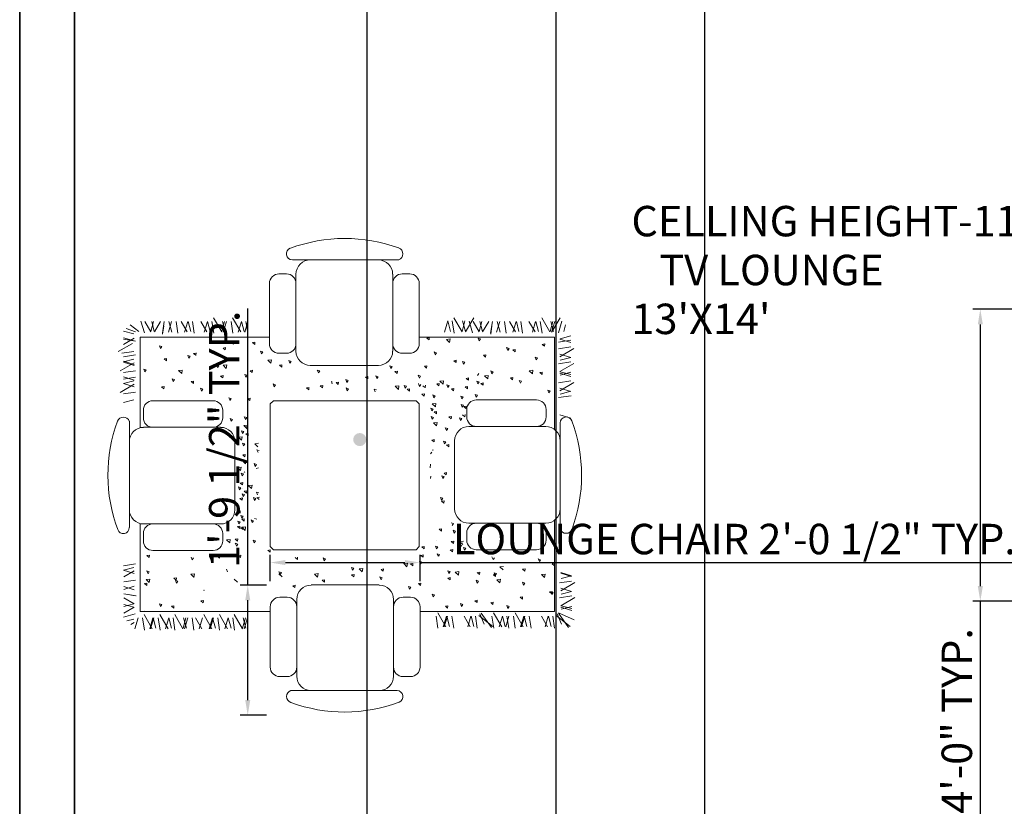
# Model space of a CAD drawing. Units: inches. Extents: x 1265 to 2734, y 1741 to 2595.
# Tile 3 of 10: x 2329 to 2490, y 2165 to 2294. Entities that reach past the tile are written whole.
import ezdxf

# ---------------------------------------------------------------- set-up
doc = ezdxf.new("R2010")
doc.units = ezdxf.units.IN
doc.header["$LTSCALE"] = 0.1
for name, color, linetype, lineweight in [('A-ANNO-DIMS', 2, 'Continuous', 18), ('A-ANNO-TEXT', 7, 'Continuous', 18), ('A-AREA-IDEN', 7, 'Continuous', 18), ('A-FURN-PATT', 252, 'Continuous', 13), ('A-WALL', 7, 'Continuous', 35), ('C-PROP', 7, 'Continuous', 35), ('Furniture', 8, 'Continuous', 15)]:
    doc.layers.add(name, color=color, linetype=linetype, lineweight=lineweight)
doc.styles.get("Standard").update_dxf_attribs({"font": 'arial.ttf', "height": 5})
doc.dimstyles.new('ISO-25', dxfattribs={"dimtxt": 5, "dimasz": 2.5, "dimexe": 1.25, "dimexo": 0.625, "dimtad": 1, "dimlunit": 3, "dimtxsty": 'Standard', "dimcen": 2.5, "dimadec": 0, "dimazin": 0, "dimtfac": 1, "dimtmove": 0, "dimatfit": 3, "dimfxl": 1, "dimarcsym": 0})

# ---------------------------------------------------------------- blocks, each defined once
blk = doc.blocks.new('CHAIR-LOUNGE')
for p, q in [((6.72, 20.87), (17.9, 20.87)), ((1.57, 18.86), (2.79, 18.86)), ((4.36, 5.87), (4.36, 18.51)), ((20.25, 18.51), (20.25, 5.87)), ((21.82, 18.86), (23.04, 18.86)), ((0, 7.39), (0, 17.29)), ((4.36, 17.29), (4.36, 7.39)), ((20.25, 7.39), (20.25, 17.29)), ((24.61, 17.29), (24.61, 7.39)), ((2.79, 5.82), (1.57, 5.82)), ((23.04, 5.82), (21.82, 5.82)), ((3.38, 3.52), (20.25, 3.52)), ((17.9, 3.52), (6.72, 3.52)), ((20.25, 3.52), (20.84, 3.52))]:
    blk.add_line(p, q)
for centre, radius, start, end in [((6.72, 18.51), 2.35, 90, 180), ((17.9, 18.51), 2.35, 0, 90), ((1.57, 17.29), 1.57, 90, 180), ((2.79, 17.29), 1.57, 0, 90), ((21.82, 17.29), 1.57, 90, 180), ((23.04, 17.29), 1.57, 0, 90), ((1.57, 7.39), 1.57, 180, 270), ((2.79, 7.39), 1.57, 270, 0), ((21.82, 7.39), 1.57, 180, 270), ((23.04, 7.39), 1.57, 270, 0), ((6.72, 5.87), 2.35, 180, 270), ((17.9, 5.87), 2.35, 270, 0), ((3.74, 2.54), 1.04, 110.0456, 249.9544), ((20.84, 2.53), 0.986, 290.3611, 90), ((12.21, 25.77), 25.77, 249.9544, 290.3611)]:
    blk.add_arc(centre, radius, start, end)
blk = doc.blocks.new('*D32')
at = {"layer": 'A-ANNO-DIMS', "color": 0, "lineweight": -2, "transparency": 16777216}
for p, q in [((2369.76, 2201.71), (2369.76, 2206.02)), ((2372.26, 2204.77), (2391.87, 2204.77)), ((2394.37, 2201.71), (2394.37, 2206.02)), ((2394.37, 2204.77), (2495.13, 2204.77))]:
    blk.add_line(p, q, dxfattribs=at)
at = {"layer": 'A-ANNO-DIMS', "color": 0, "lineweight": 100, "transparency": 16777216}
for points in [[(2372.26, 2205.19), (2372.26, 2204.36), (2369.76, 2204.77)], [(2391.87, 2205.19), (2391.87, 2204.36), (2394.37, 2204.77)]]:
    blk.add_solid(points, dxfattribs=at)
at = {"layer": 'Defpoints', "color": 0, "lineweight": 100, "transparency": 16777216}
for p in [(2394.37, 2204.77), (2369.76, 2201.08), (2394.37, 2201.08)]:
    blk.add_point(p, dxfattribs=at)
at = {"layer": 'A-ANNO-DIMS', "color": 0, "transparency": 16777216, "insert": (2446, 2207.99), "char_height": 5, "attachment_point": 5}
blk.add_mtext('LOUNGE CHAIR 2\'-0 1/2" TYP.', dxfattribs=at)
blk = doc.blocks.new('*D33')
at = {"layer": 'A-ANNO-DIMS', "color": 0, "lineweight": -2, "transparency": 16777216}
for p, q in [((2366.06, 2201.08), (2366.06, 2246.49)), ((2369.13, 2201.08), (2364.81, 2201.08)), ((2366.06, 2182.18), (2366.06, 2198.58)), ((2369.13, 2179.68), (2364.81, 2179.68))]:
    blk.add_line(p, q, dxfattribs=at)
at = {"layer": 'A-ANNO-DIMS', "color": 0, "lineweight": 100, "transparency": 16777216}
for points in [[(2365.65, 2198.58), (2366.48, 2198.58), (2366.06, 2201.08)], [(2365.65, 2182.18), (2366.48, 2182.18), (2366.06, 2179.68)]]:
    blk.add_solid(points, dxfattribs=at)
at = {"layer": 'Defpoints', "color": 0, "lineweight": 100, "transparency": 16777216}
for p in [(2366.06, 2201.08), (2369.76, 2201.08), (2369.76, 2179.68)]:
    blk.add_point(p, dxfattribs=at)
at = {"layer": 'A-ANNO-DIMS', "color": 0, "transparency": 16777216, "insert": (2362.85, 2225.04), "char_height": 5, "attachment_point": 5, "rotation": 90}
blk.add_mtext('1\'-9 1/2" TYP.', dxfattribs=at)
blk = doc.blocks.new('*D36')
at = {"layer": 'A-ANNO-DIMS', "color": 0, "lineweight": -2, "transparency": 16777216}
for p, q in [((2492.98, 2246.41), (2485.15, 2246.41)), ((2486.4, 2243.91), (2486.4, 2200.91)), ((2492.98, 2198.41), (2485.15, 2198.41)), ((2486.4, 2198.41), (2486.4, 2131.39))]:
    blk.add_line(p, q, dxfattribs=at)
at = {"layer": 'A-ANNO-DIMS', "color": 0, "lineweight": 100, "transparency": 16777216}
for points in [[(2485.99, 2243.91), (2486.82, 2243.91), (2486.4, 2246.41)], [(2485.99, 2200.91), (2486.82, 2200.91), (2486.4, 2198.41)]]:
    blk.add_solid(points, dxfattribs=at)
at = {"layer": 'Defpoints', "color": 0, "lineweight": 100, "transparency": 16777216}
for p in [(2493.6, 2246.41), (2486.4, 2198.41), (2493.6, 2198.41)]:
    blk.add_point(p, dxfattribs=at)
at = {"layer": 'A-ANNO-DIMS', "color": 0, "transparency": 16777216, "insert": (2483.19, 2163.65), "char_height": 5, "attachment_point": 5, "rotation": 90}
blk.add_mtext('WINDOW 4\'-0" TYP.', dxfattribs=at)
blk = doc.blocks.new('*D42')
at = {"layer": 'A-ANNO-DIMS', "color": 0, "lineweight": -2, "transparency": 16777216}
for p, q in [((2328.6, 1822.68), (2328.6, 2585.16)), ((2521.32, 1822.68), (2521.32, 2585.16)), ((2331.1, 2583.91), (2518.82, 2583.91))]:
    blk.add_line(p, q, dxfattribs=at)
at = {"layer": 'A-ANNO-DIMS', "color": 0, "lineweight": 100, "transparency": 16777216}
for points in [[(2331.1, 2584.32), (2331.1, 2583.49), (2328.6, 2583.91)], [(2518.82, 2584.32), (2518.82, 2583.49), (2521.32, 2583.91)]]:
    blk.add_solid(points, dxfattribs=at)
at = {"layer": 'Defpoints', "color": 0, "lineweight": 100, "transparency": 16777216}
for p in [(2521.32, 2583.91), (2328.6, 1822.06), (2521.32, 1822.06)]:
    blk.add_point(p, dxfattribs=at)
at = {"layer": 'A-ANNO-DIMS', "color": 0, "transparency": 16777216, "insert": (2424.96, 2587.12), "char_height": 5, "attachment_point": 5}
blk.add_mtext('16\'-0 1/2"', dxfattribs=at)
blk = doc.blocks.new('*D43')
at = {"layer": 'A-ANNO-DIMS', "color": 0, "lineweight": -2, "transparency": 16777216}
for p, q in [((2337.6, 2308.03), (2337.6, 1744.16)), ((2441.1, 2308.03), (2441.1, 1744.16)), ((2340.1, 1745.41), (2438.6, 1745.41))]:
    blk.add_line(p, q, dxfattribs=at)
at = {"layer": 'A-ANNO-DIMS', "color": 0, "lineweight": 100, "transparency": 16777216}
for points in [[(2340.1, 1745.82), (2340.1, 1744.99), (2337.6, 1745.41)], [(2438.6, 1745.82), (2438.6, 1744.99), (2441.1, 1745.41)]]:
    blk.add_solid(points, dxfattribs=at)
at = {"layer": 'Defpoints', "color": 0, "lineweight": 100, "transparency": 16777216}
for p in [(2337.6, 2308.66), (2441.1, 2308.66), (2441.1, 1745.41)]:
    blk.add_point(p, dxfattribs=at)
at = {"layer": 'A-ANNO-DIMS', "color": 0, "transparency": 16777216, "insert": (2389.35, 1748.62), "char_height": 5, "attachment_point": 5}
blk.add_mtext('8\'-7 1/2"', dxfattribs=at)
blk = doc.blocks.new('*D45')
at = {"layer": 'A-ANNO-DIMS', "color": 0, "lineweight": -2, "transparency": 16777216}
for p, q in [((2416.67, 2477.91), (2416.67, 1744.16)), ((2385.6, 2477.53), (2385.6, 1744.16)), ((2388.1, 1745.41), (2414.17, 1745.41))]:
    blk.add_line(p, q, dxfattribs=at)
at = {"layer": 'A-ANNO-DIMS', "color": 0, "lineweight": 100, "transparency": 16777216}
for points in [[(2388.1, 1745.82), (2388.1, 1744.99), (2385.6, 1745.41)], [(2414.17, 1745.82), (2414.17, 1744.99), (2416.67, 1745.41)]]:
    blk.add_solid(points, dxfattribs=at)
at = {"layer": 'Defpoints', "color": 0, "lineweight": 100, "transparency": 16777216}
for p in [(2385.6, 2478.16), (2416.67, 2478.54), (2416.67, 1745.41)]:
    blk.add_point(p, dxfattribs=at)
at = {"layer": 'A-ANNO-DIMS', "color": 0, "transparency": 16777216, "insert": (2401.14, 1748.54), "char_height": 5, "attachment_point": 5}
blk.add_mtext('2\'-7"', dxfattribs=at)

msp = doc.modelspace()

# ---------------------------------------------------------------- hatches: boundary and pattern name
at = {"layer": 'A-FURN-PATT'}
msp.add_hatch(color=256, dxfattribs=at).paths.add_polyline_path([(2385.543, 2224.98, 1), (2383.383, 2224.98, 1)])

# ---------------------------------------------------------------- linework, layer by layer
at = {"layer": 'A-WALL'}
msp.add_line((2337.602, 2140.657), (2337.602, 2308.657), dxfattribs=at)
at = {"layer": 'C-PROP'}
msp.add_line((2328.602, 1786.657), (2328.602, 2542.657), dxfattribs=at)
at = {"layer": 'Furniture'}
for p, q in [((2360.445, 2244.981), (2361.794, 2242.659)), ((2363.57, 2244.981), (2364.919, 2242.659)), ((2399.915, 2244.981), (2401.264, 2242.659)), ((2403.197, 2244.981), (2401.847, 2242.659)), ((2414.364, 2244.981), (2415.714, 2242.659)), ((2417.379, 2244.981), (2416.03, 2242.659)), ((2346.729, 2243.841), (2348.199, 2242.736)), ((2348.501, 2244.434), (2349.08, 2242.515)), ((2349.158, 2244.364), (2350.149, 2242.659)), ((2350.594, 2244.368), (2350.165, 2242.736)), ((2350.287, 2244.367), (2350.716, 2242.736)), ((2351.727, 2244.371), (2350.732, 2242.659)), ((2352.333, 2244.373), (2352.042, 2242.444)), ((2352.254, 2243.646), (2352.051, 2242.304)), ((2353.545, 2244.376), (2353.026, 2242.655)), ((2353.092, 2244.375), (2353.611, 2242.655)), ((2354.303, 2244.378), (2354.595, 2242.444)), ((2355.135, 2244.38), (2356.135, 2242.659)), ((2356.223, 2244.383), (2355.702, 2242.655)), ((2356.269, 2244.383), (2356.702, 2242.736)), ((2356.978, 2244.385), (2357.271, 2242.444)), ((2358.343, 2244.389), (2359.348, 2242.659)), ((2359.439, 2244.392), (2358.915, 2242.655)), ((2359.48, 2244.392), (2359.915, 2242.736)), ((2360.19, 2244.394), (2360.484, 2242.444)), ((2362.248, 2244.399), (2361.81, 2242.736)), ((2361.924, 2244.398), (2362.361, 2242.736)), ((2362.567, 2244.4), (2362.04, 2242.655)), ((2363.314, 2244.402), (2363.609, 2242.444)), ((2365.014, 2244.406), (2364.486, 2242.655)), ((2365.047, 2244.406), (2365.486, 2242.736)), ((2366.102, 2244.409), (2365.573, 2242.655)), ((2365.758, 2244.408), (2366.055, 2242.444)), ((2398.941, 2244.497), (2398.385, 2242.655)), ((2398.922, 2244.497), (2399.385, 2242.736)), ((2399.644, 2244.499), (2399.954, 2242.444)), ((2401.745, 2244.504), (2401.28, 2242.736)), ((2401.366, 2244.503), (2401.831, 2242.736)), ((2402.421, 2244.434), (2403, 2242.515)), ((2403.078, 2244.364), (2404.069, 2242.659)), ((2404.514, 2244.368), (2404.085, 2242.736)), ((2404.207, 2244.367), (2404.636, 2242.736)), ((2405.647, 2244.371), (2404.652, 2242.659)), ((2406.253, 2244.373), (2405.962, 2242.444)), ((2406.173, 2243.646), (2405.971, 2242.304)), ((2407.465, 2244.376), (2406.945, 2242.655)), ((2407.012, 2244.375), (2407.531, 2242.655)), ((2408.223, 2244.378), (2408.514, 2242.444)), ((2409.055, 2244.38), (2410.055, 2242.659)), ((2410.143, 2244.383), (2409.622, 2242.655)), ((2410.188, 2244.383), (2410.622, 2242.736)), ((2410.898, 2244.385), (2411.191, 2242.444)), ((2412.263, 2244.389), (2413.268, 2242.659)), ((2413.359, 2244.392), (2412.835, 2242.655)), ((2413.399, 2244.392), (2413.835, 2242.736)), ((2414.11, 2244.394), (2414.404, 2242.444)), ((2416.167, 2244.399), (2415.73, 2242.736)), ((2415.844, 2244.398), (2416.281, 2242.736)), ((2416.486, 2244.4), (2415.96, 2242.655)), ((2417.678, 2244.434), (2417.099, 2242.515)), ((2418.27, 2243.841), (2417.979, 2242.736)), ((2345.638, 2242.806), (2347.329, 2242.361)), ((2345.638, 2241.719), (2347.409, 2241.184)), ((2346.12, 2243.232), (2347.632, 2242.659)), ((2348.415, 2226.932), (2348.415, 2241.805)), ((2348.415, 2241.805), (2369.627, 2241.805)), ((2394.237, 2241.805), (2416.453, 2241.805)), ((2395.892, 2241.73), (2395.489, 2241.656)), ((2395.857, 2241.348), (2395.89, 2241.732)), ((2406.546, 2241.802), (2406.542, 2241.805)), ((2406.546, 2241.801), (2406.546, 2241.805)), ((2416.453, 2241.805), (2416.453, 2226.644)), ((2419.139, 2242.007), (2417.402, 2241.55)), ((2344.802, 2239.433), (2347.123, 2240.783)), ((2345.636, 2241.471), (2347.621, 2241.171)), ((2345.641, 2240.592), (2347.406, 2241.618)), ((2351.957, 2240.253), (2351.568, 2240.384)), ((2351.742, 2239.934), (2351.569, 2240.385)), ((2351.741, 2239.933), (2351.957, 2240.253)), ((2363.665, 2240.644), (2363.492, 2241.094)), ((2363.881, 2240.963), (2363.492, 2241.093)), ((2363.665, 2240.643), (2363.881, 2240.963)), ((2367.219, 2240.607), (2366.849, 2240.918)), ((2367.254, 2240.989), (2366.85, 2240.915)), ((2367.219, 2240.606), (2367.252, 2240.991)), ((2395.857, 2241.349), (2395.487, 2241.659)), ((2399.301, 2241.521), (2398.689, 2241.45)), ((2399.212, 2240.949), (2398.69, 2241.45)), ((2399.212, 2240.948), (2399.301, 2241.521)), ((2404.102, 2241.207), (2403.929, 2241.658)), ((2404.317, 2241.526), (2403.929, 2241.656)), ((2404.102, 2241.206), (2404.318, 2241.526)), ((2414.815, 2240.305), (2414.445, 2240.615)), ((2414.85, 2240.686), (2414.446, 2240.612)), ((2414.814, 2240.304), (2414.848, 2240.688)), ((2419.141, 2241.288), (2417.111, 2240.981)), ((2419.144, 2240.201), (2417.111, 2239.894)), ((2419.142, 2240.914), (2417.322, 2241.464)), ((2345.371, 2239.176), (2347.338, 2239.473)), ((2345.647, 2238.585), (2347.621, 2238.883)), ((2356.408, 2238.368), (2356.235, 2238.819)), ((2356.623, 2238.687), (2356.235, 2238.818)), ((2356.408, 2238.367), (2356.624, 2238.688)), ((2357.538, 2238.822), (2357.168, 2239.132)), ((2357.573, 2239.203), (2357.17, 2239.129)), ((2357.538, 2238.82), (2357.571, 2239.205)), ((2362.378, 2239.715), (2362.009, 2240.025)), ((2362.413, 2240.096), (2362.01, 2240.022)), ((2362.378, 2239.713), (2362.412, 2240.098)), ((2368.547, 2239.397), (2368.158, 2239.527)), ((2368.332, 2239.078), (2368.159, 2239.529)), ((2368.331, 2239.077), (2368.547, 2239.397)), ((2397.06, 2239.25), (2396.671, 2239.381)), ((2396.845, 2238.932), (2396.672, 2239.382)), ((2396.844, 2238.931), (2397.06, 2239.251)), ((2405.134, 2238.519), (2404.764, 2238.83)), ((2405.169, 2238.9), (2404.766, 2238.826)), ((2405.134, 2238.518), (2405.167, 2238.903)), ((2408.984, 2239.96), (2408.595, 2240.091)), ((2408.769, 2239.641), (2408.596, 2240.092)), ((2408.768, 2239.64), (2408.984, 2239.96)), ((2409.974, 2239.412), (2409.605, 2239.722)), ((2410.009, 2239.793), (2409.606, 2239.719)), ((2409.974, 2239.411), (2410.008, 2239.795)), ((2413.65, 2238.394), (2413.261, 2238.525)), ((2413.435, 2238.076), (2413.262, 2238.526)), ((2419.149, 2238.466), (2417.322, 2239.018)), ((2419.647, 2239.934), (2417.326, 2238.585)), ((2345.084, 2236.262), (2347.406, 2237.611)), ((2345.649, 2237.736), (2347.329, 2238.178)), ((2345.649, 2237.845), (2347.409, 2237.314)), ((2345.649, 2237.709), (2347.409, 2237.178)), ((2352.698, 2237.929), (2352.328, 2238.239)), ((2352.733, 2238.31), (2352.329, 2238.236)), ((2352.697, 2237.928), (2352.731, 2238.312)), ((2361.29, 2237.122), (2360.901, 2237.252)), ((2361.075, 2236.803), (2360.902, 2237.253)), ((2361.074, 2236.802), (2361.29, 2237.122)), ((2362.633, 2237.255), (2362.022, 2237.184)), ((2362.544, 2236.683), (2362.022, 2237.184)), ((2362.544, 2236.683), (2362.633, 2237.255)), ((2369.966, 2238.108), (2369.355, 2238.037)), ((2369.878, 2237.536), (2369.356, 2238.037)), ((2369.878, 2237.536), (2369.967, 2238.108)), ((2371.655, 2236.885), (2371.286, 2237.195)), ((2371.69, 2237.266), (2371.287, 2237.192)), ((2371.655, 2236.884), (2371.689, 2237.268)), ((2373.213, 2237.831), (2372.824, 2237.962)), ((2372.998, 2237.512), (2372.825, 2237.963)), ((2372.997, 2237.511), (2373.213, 2237.831)), ((2389.803, 2236.975), (2389.414, 2237.106)), ((2389.588, 2236.656), (2389.415, 2237.107)), ((2389.587, 2236.655), (2389.803, 2236.975)), ((2395.453, 2236.734), (2395.084, 2237.044)), ((2395.488, 2237.115), (2395.085, 2237.04)), ((2395.453, 2236.732), (2395.487, 2237.117)), ((2400.294, 2237.626), (2399.924, 2237.937)), ((2400.329, 2238.008), (2399.925, 2237.933)), ((2400.293, 2237.625), (2400.327, 2238.01)), ((2401.727, 2237.685), (2401.338, 2237.815)), ((2401.512, 2237.366), (2401.339, 2237.816)), ((2401.511, 2237.365), (2401.727, 2237.685)), ((2413.434, 2238.075), (2413.65, 2238.395)), ((2419.151, 2237.757), (2417.111, 2237.449)), ((2419.647, 2237.488), (2417.326, 2236.139)), ((2419.149, 2238.477), (2417.402, 2238.018)), ((2345.654, 2236.004), (2347.621, 2236.301)), ((2345.656, 2235.262), (2347.409, 2234.732)), ((2349.366, 2236.412), (2348.977, 2236.542)), ((2349.151, 2236.093), (2348.978, 2236.544)), ((2349.15, 2236.092), (2349.366, 2236.412)), ((2355.299, 2236.402), (2354.688, 2236.331)), ((2355.211, 2235.83), (2354.689, 2236.331)), ((2355.211, 2235.83), (2355.3, 2236.402)), ((2361.975, 2235.099), (2361.605, 2235.409)), ((2362.01, 2235.481), (2361.606, 2235.406)), ((2361.974, 2235.098), (2362.008, 2235.482)), ((2365.956, 2235.556), (2365.567, 2235.686)), ((2365.741, 2235.237), (2365.568, 2235.687)), ((2365.74, 2235.236), (2365.956, 2235.556)), ((2366.815, 2235.992), (2366.445, 2236.302)), ((2366.85, 2236.373), (2366.447, 2236.299)), ((2366.815, 2235.991), (2366.848, 2236.375)), ((2377.664, 2235.947), (2377.491, 2236.397)), ((2377.88, 2236.265), (2377.491, 2236.396)), ((2377.664, 2235.946), (2377.88, 2236.266)), ((2385.773, 2234.948), (2385.403, 2235.258)), ((2385.807, 2235.329), (2385.404, 2235.255)), ((2385.772, 2234.947), (2385.806, 2235.331)), ((2387.499, 2235.314), (2387.11, 2235.445)), ((2387.284, 2234.995), (2387.111, 2235.446)), ((2387.283, 2234.994), (2387.499, 2235.314)), ((2390.613, 2235.841), (2390.243, 2236.151)), ((2390.648, 2236.222), (2390.244, 2236.148)), ((2390.613, 2235.839), (2390.646, 2236.224)), ((2394.469, 2235.409), (2394.08, 2235.54)), ((2394.254, 2235.091), (2394.081, 2235.541)), ((2394.254, 2235.09), (2394.469, 2235.41)), ((2403.825, 2235.507), (2404.041, 2235.827)), ((2405.569, 2235.506), (2404.958, 2235.435)), ((2405.481, 2234.934), (2404.958, 2235.435)), ((2405.481, 2234.934), (2405.569, 2235.506)), ((2406.393, 2236.119), (2406.004, 2236.249)), ((2406.178, 2235.8), (2406.005, 2236.251)), ((2406.177, 2235.799), (2406.393, 2236.119)), ((2412.902, 2236.359), (2412.291, 2236.288)), ((2412.814, 2235.787), (2412.292, 2236.288)), ((2412.814, 2235.787), (2412.903, 2236.359)), ((2414.411, 2235.689), (2414.041, 2236)), ((2414.446, 2236.071), (2414.042, 2235.996)), ((2414.411, 2235.688), (2414.444, 2236.073)), ((2419.157, 2235.339), (2417.322, 2235.893)), ((2419.156, 2235.661), (2417.402, 2236.122)), ((2419.155, 2236.033), (2417.402, 2235.572)), ((2345.084, 2232.729), (2347.406, 2234.079)), ((2345.657, 2234.918), (2347.621, 2235.214)), ((2345.658, 2234.206), (2347.329, 2234.645)), ((2345.658, 2234.174), (2347.409, 2233.645)), ((2352.329, 2233.695), (2351.926, 2233.621)), ((2352.294, 2233.312), (2352.327, 2233.697)), ((2353.817, 2234.527), (2353.644, 2234.978)), ((2354.033, 2234.846), (2353.644, 2234.977)), ((2353.817, 2234.526), (2354.033, 2234.846)), ((2357.134, 2234.206), (2356.765, 2234.516)), ((2357.169, 2234.588), (2356.766, 2234.513)), ((2357.134, 2234.205), (2357.168, 2234.59)), ((2370.622, 2233.99), (2370.233, 2234.121)), ((2370.407, 2233.671), (2370.234, 2234.122)), ((2370.407, 2233.67), (2370.622, 2233.99)), ((2378.344, 2233.478), (2377.974, 2233.788)), ((2378.379, 2233.86), (2377.975, 2233.785)), ((2378.344, 2233.477), (2378.377, 2233.861)), ((2379.957, 2234.487), (2379.805, 2234.538)), ((2379.957, 2234.145), (2379.806, 2234.539)), ((2380.932, 2234.055), (2380.563, 2234.365)), ((2380.967, 2234.436), (2380.564, 2234.362)), ((2380.932, 2234.054), (2380.966, 2234.438)), ((2382.546, 2234.7), (2382.157, 2234.83)), ((2382.331, 2234.381), (2382.158, 2234.831)), ((2382.33, 2234.38), (2382.546, 2234.7)), ((2390.902, 2233.8), (2390.291, 2233.729)), ((2390.814, 2233.228), (2390.291, 2233.729)), ((2390.813, 2233.227), (2390.902, 2233.8)), ((2392.165, 2233.748), (2391.776, 2233.879)), ((2391.95, 2233.43), (2391.777, 2233.88)), ((2391.95, 2233.429), (2392.165, 2233.749)), ((2394.302, 2233.722), (2394.129, 2234.172)), ((2394.302, 2233.721), (2394.517, 2234.041)), ((2395.216, 2233.509), (2394.846, 2233.819)), ((2395.215, 2233.508), (2395.249, 2233.893)), ((2397.468, 2233.825), (2397.098, 2234.135)), ((2397.502, 2234.206), (2397.099, 2234.132)), ((2397.467, 2233.824), (2397.501, 2234.209)), ((2398.235, 2234.653), (2397.624, 2234.582)), ((2398.147, 2234.081), (2397.625, 2234.582)), ((2398.147, 2234.081), (2398.236, 2234.653)), ((2399.136, 2233.844), (2398.747, 2233.974)), ((2398.921, 2233.525), (2398.748, 2233.975)), ((2398.92, 2233.524), (2399.136, 2233.844)), ((2402.142, 2233.327), (2401.772, 2233.637)), ((2402.177, 2233.708), (2401.773, 2233.634)), ((2402.308, 2234.718), (2401.938, 2235.028)), ((2402.343, 2235.099), (2401.939, 2235.025)), ((2402.141, 2233.326), (2402.175, 2233.71)), ((2402.308, 2234.717), (2402.341, 2235.101)), ((2404.089, 2234.458), (2403.7, 2234.588)), ((2403.874, 2234.139), (2403.701, 2234.59)), ((2403.873, 2234.138), (2404.089, 2234.458)), ((2404.73, 2233.904), (2404.36, 2234.214)), ((2404.765, 2234.285), (2404.362, 2234.211)), ((2404.73, 2233.902), (2404.763, 2234.287)), ((2409.57, 2234.797), (2409.201, 2235.107)), ((2409.605, 2235.178), (2409.202, 2235.103)), ((2409.57, 2234.795), (2409.604, 2235.18)), ((2411.059, 2234.553), (2410.67, 2234.684)), ((2410.844, 2234.234), (2410.671, 2234.685)), ((2410.843, 2234.233), (2411.059, 2234.554)), ((2419.159, 2234.633), (2417.111, 2234.324)), ((2419.647, 2234.363), (2417.326, 2233.014)), ((2345.663, 2232.473), (2347.621, 2232.769)), ((2352.294, 2233.313), (2351.924, 2233.623)), ((2358.699, 2233.281), (2358.31, 2233.411)), ((2358.484, 2232.962), (2358.311, 2233.412)), ((2358.483, 2232.961), (2358.699, 2233.281)), ((2376.092, 2233.162), (2375.722, 2233.472)), ((2376.127, 2233.544), (2375.723, 2233.469)), ((2376.092, 2233.161), (2376.125, 2233.545)), ((2382.594, 2233.331), (2382.205, 2233.461)), ((2382.379, 2233.012), (2382.206, 2233.462)), ((2382.378, 2233.011), (2382.594, 2233.331)), ((2387.212, 2233.134), (2386.823, 2233.264)), ((2386.997, 2232.815), (2386.824, 2233.266)), ((2392.627, 2232.932), (2392.258, 2233.243)), ((2392.662, 2233.314), (2392.259, 2233.239)), ((2392.627, 2232.931), (2392.661, 2233.316)), ((2395.049, 2232.118), (2394.68, 2232.428)), ((2395.084, 2232.499), (2394.681, 2232.425)), ((2395.049, 2232.117), (2395.083, 2232.501)), ((2396.832, 2232.183), (2396.443, 2232.313)), ((2396.617, 2231.864), (2396.444, 2232.314)), ((2396.616, 2231.863), (2396.832, 2232.183)), ((2399.89, 2233.011), (2399.52, 2233.321)), ((2399.925, 2233.392), (2399.521, 2233.318)), ((2399.889, 2233.01), (2399.923, 2233.394)), ((2401.45, 2231.986), (2401.061, 2232.116)), ((2401.235, 2231.667), (2401.062, 2232.118)), ((2403.802, 2232.278), (2403.413, 2232.408)), ((2403.587, 2231.959), (2403.414, 2232.41)), ((2403.586, 2231.958), (2403.802, 2232.278)), ((2415.726, 2232.988), (2415.337, 2233.118)), ((2415.511, 2232.669), (2415.338, 2233.119)), ((2415.51, 2232.668), (2415.726, 2232.988)), ((2419.165, 2232.188), (2417.111, 2231.878)), ((2419.164, 2232.891), (2417.322, 2233.447)), ((2419.163, 2232.91), (2417.402, 2232.447)), ((2345.667, 2231.083), (2347.329, 2231.52)), ((2363.365, 2231.715), (2362.976, 2231.845)), ((2363.15, 2231.396), (2362.977, 2231.846)), ((2363.149, 2231.395), (2363.365, 2231.715)), ((2366.411, 2231.376), (2366.041, 2231.687)), ((2366.446, 2231.758), (2366.043, 2231.683)), ((2366.411, 2231.375), (2366.445, 2231.76)), ((2369.763, 2230.843), (2370.273, 2231.353)), ((2369.763, 2207.396), (2369.763, 2230.843)), ((2370.273, 2231.353), (2393.72, 2231.353)), ((2393.72, 2231.353), (2394.23, 2230.843)), ((2394.23, 2230.843), (2394.23, 2207.396)), ((2396.984, 2230.924), (2396.373, 2230.853)), ((2396.896, 2230.351), (2396.373, 2230.853)), ((2396.895, 2230.351), (2396.984, 2230.923)), ((2401.498, 2230.617), (2401.109, 2230.747)), ((2401.283, 2230.298), (2401.11, 2230.749)), ((2401.234, 2231.666), (2401.45, 2231.986)), ((2401.282, 2230.297), (2401.498, 2230.617)), ((2401.904, 2230.103), (2401.534, 2230.413)), ((2401.939, 2230.484), (2401.536, 2230.409)), ((2401.904, 2230.101), (2401.937, 2230.486)), ((2396.545, 2230.003), (2396.156, 2230.133)), ((2396.33, 2229.684), (2396.157, 2230.134)), ((2396.329, 2229.683), (2396.545, 2230.003)), ((2397.064, 2229.21), (2396.694, 2229.52)), ((2397.099, 2229.591), (2396.695, 2229.516)), ((2397.063, 2229.208), (2397.097, 2229.593)), ((2399.486, 2228.394), (2399.519, 2228.779)), ((2401.738, 2228.711), (2401.368, 2229.021)), ((2401.738, 2228.71), (2401.771, 2229.095)), ((2419.149, 2228.482), (2417.322, 2229.033)), ((2363.323, 2227.984), (2363.15, 2228.435)), ((2363.538, 2228.303), (2363.15, 2228.433)), ((2363.323, 2227.983), (2363.539, 2228.303)), ((2366.042, 2227.336), (2365.431, 2227.265)), ((2365.954, 2226.764), (2365.432, 2227.265)), ((2365.89, 2228.595), (2365.501, 2228.725)), ((2365.675, 2228.276), (2365.502, 2228.727)), ((2365.675, 2228.275), (2365.89, 2228.595)), ((2365.954, 2226.763), (2366.043, 2227.336)), ((2396.593, 2228.634), (2396.204, 2228.764)), ((2396.378, 2228.315), (2396.205, 2228.765)), ((2396.377, 2228.314), (2396.593, 2228.634)), ((2397.17, 2227.786), (2396.559, 2227.714)), ((2397.082, 2227.213), (2396.56, 2227.714)), ((2397.082, 2227.213), (2397.171, 2227.785)), ((2399.486, 2228.395), (2399.116, 2228.706)), ((2399.521, 2228.777), (2399.117, 2228.702)), ((2401.211, 2228.437), (2400.822, 2228.567)), ((2400.996, 2228.118), (2400.823, 2228.569)), ((2400.995, 2228.117), (2401.211, 2228.437)), ((2365.441, 2226.308), (2365.052, 2226.438)), ((2365.226, 2225.989), (2365.053, 2226.44)), ((2365.225, 2225.988), (2365.441, 2226.308)), ((2366.007, 2226.761), (2365.638, 2227.071)), ((2366.042, 2227.142), (2365.639, 2227.068)), ((2366.122, 2225.622), (2365.753, 2225.932)), ((2366.157, 2226.003), (2365.754, 2225.929)), ((2366.007, 2226.76), (2366.041, 2227.144)), ((2366.122, 2225.621), (2366.156, 2226.005)), ((2398.907, 2226.776), (2398.518, 2226.906)), ((2398.692, 2226.457), (2398.519, 2226.908)), ((2398.691, 2226.456), (2398.907, 2226.776)), ((2365.14, 2225.44), (2364.529, 2225.368)), ((2365.052, 2224.867), (2364.529, 2225.369)), ((2365.051, 2224.867), (2365.14, 2225.439)), ((2365.566, 2224.265), (2365.177, 2224.396)), ((2365.351, 2223.946), (2365.178, 2224.397)), ((2365.35, 2223.945), (2365.566, 2224.265)), ((2367.836, 2224.373), (2367.225, 2224.302)), ((2367.748, 2223.801), (2367.225, 2224.302)), ((2396.66, 2224.594), (2396.29, 2224.904)), ((2396.695, 2224.975), (2396.291, 2224.901)), ((2396.66, 2224.593), (2396.693, 2224.977)), ((2398.62, 2224.596), (2398.231, 2224.726)), ((2398.405, 2224.277), (2398.232, 2224.727)), ((2398.405, 2224.276), (2398.62, 2224.596)), ((2399.082, 2223.78), (2398.712, 2224.09)), ((2399.117, 2224.161), (2398.714, 2224.087)), ((2399.082, 2223.778), (2399.116, 2224.163)), ((2365.604, 2222.145), (2365.234, 2222.455)), ((2365.638, 2222.527), (2365.235, 2222.452)), ((2365.603, 2222.144), (2365.637, 2222.529)), ((2367.966, 2223.188), (2367.577, 2223.319)), ((2367.751, 2222.869), (2367.578, 2223.32)), ((2396.101, 2222.615), (2396.316, 2222.935)), ((2396.494, 2223.203), (2396.401, 2223.281)), ((2396.493, 2223.202), (2396.5, 2223.281)), ((2365.719, 2221.006), (2365.349, 2221.317)), ((2365.753, 2221.388), (2365.35, 2221.313)), ((2365.718, 2221.005), (2365.752, 2221.39)), ((2367.516, 2220.901), (2367.127, 2221.032)), ((2367.301, 2220.582), (2367.128, 2221.033)), ((2367.3, 2220.581), (2367.516, 2220.901)), ((2396.017, 2220.345), (2396.106, 2220.918)), ((2364.977, 2220.468), (2364.366, 2220.397)), ((2364.889, 2219.896), (2364.367, 2220.397)), ((2364.889, 2219.896), (2364.978, 2220.468)), ((2365.375, 2219.347), (2364.986, 2219.478)), ((2365.16, 2219.028), (2364.987, 2219.479)), ((2365.159, 2219.027), (2365.375, 2219.347)), ((2365.552, 2219.615), (2365.46, 2219.693)), ((2365.552, 2219.614), (2365.559, 2219.693)), ((2367.839, 2220.313), (2367.436, 2220.238)), ((2398.678, 2219.164), (2398.309, 2219.474)), ((2398.713, 2219.545), (2398.31, 2219.471)), ((2398.678, 2219.163), (2398.712, 2219.548)), ((2365.2, 2217.53), (2364.83, 2217.84)), ((2365.235, 2217.911), (2364.831, 2217.837)), ((2365.199, 2217.528), (2365.233, 2217.913)), ((2366.771, 2217.505), (2366.16, 2217.434)), ((2366.683, 2216.933), (2366.771, 2217.505)), ((2396.09, 2218.586), (2396.123, 2218.971)), ((2398.344, 2218.897), (2397.955, 2219.027)), ((2398.129, 2218.578), (2397.956, 2219.029)), ((2398.128, 2218.577), (2398.344, 2218.897)), ((2364.925, 2217.06), (2364.536, 2217.191)), ((2364.71, 2216.741), (2364.537, 2217.192)), ((2364.71, 2216.74), (2364.925, 2217.06)), ((2365.313, 2215.614), (2365.14, 2216.065)), ((2365.528, 2215.933), (2365.14, 2216.064)), ((2365.265, 2216.982), (2365.269, 2216.989)), ((2365.313, 2215.613), (2365.529, 2215.934)), ((2365.863, 2216.201), (2365.493, 2216.511)), ((2365.898, 2216.582), (2365.494, 2216.507)), ((2365.863, 2216.199), (2365.896, 2216.584)), ((2366.683, 2216.933), (2366.16, 2217.434)), ((2367.665, 2215.906), (2367.492, 2216.357)), ((2367.88, 2216.225), (2367.492, 2216.356)), ((2365.149, 2215), (2364.779, 2215.31)), ((2365.183, 2215.381), (2364.78, 2215.307)), ((2365.148, 2214.998), (2365.182, 2215.383)), ((2367.187, 2214.99), (2367.014, 2215.441)), ((2367.402, 2215.309), (2367.014, 2215.44)), ((2367.187, 2214.989), (2367.403, 2215.31)), ((2367.949, 2215.125), (2367.579, 2215.435)), ((2367.983, 2215.507), (2367.58, 2215.432)), ((2398.105, 2215.348), (2397.716, 2215.478)), ((2397.89, 2215.029), (2397.717, 2215.48)), ((2397.889, 2215.028), (2398.105, 2215.348)), ((2398.275, 2214.549), (2397.905, 2214.859)), ((2398.309, 2214.93), (2397.906, 2214.855)), ((2398.274, 2214.547), (2398.308, 2214.932)), ((2364.796, 2212.914), (2364.426, 2213.224)), ((2364.831, 2213.296), (2364.427, 2213.221)), ((2364.796, 2212.913), (2364.829, 2213.297)), ((2348.415, 2208.895), (2348.415, 2211.179)), ((2364.812, 2211.468), (2364.423, 2211.599)), ((2364.597, 2211.149), (2364.424, 2211.6)), ((2364.596, 2211.148), (2364.812, 2211.468)), ((2365.29, 2212.384), (2364.901, 2212.515)), ((2365.075, 2212.065), (2364.902, 2212.516)), ((2365.074, 2212.064), (2365.29, 2212.385)), ((2365.459, 2211.585), (2365.089, 2211.895)), ((2365.494, 2211.966), (2365.091, 2211.892)), ((2365.459, 2211.584), (2365.493, 2211.968)), ((2367.001, 2211.653), (2366.612, 2211.784)), ((2366.786, 2211.334), (2366.613, 2211.785)), ((2366.785, 2211.333), (2367.001, 2211.653)), ((2367.556, 2211.895), (2367.167, 2212.026)), ((2399.877, 2211.175), (2399.488, 2211.305)), ((2399.662, 2210.855), (2399.877, 2211.175)), ((2416.453, 2211.723), (2416.453, 2208.895)), ((2364.745, 2210.384), (2364.375, 2210.694)), ((2364.78, 2210.765), (2364.376, 2210.691)), ((2364.744, 2210.383), (2364.778, 2210.767)), ((2365.293, 2210.194), (2364.923, 2210.504)), ((2365.328, 2210.575), (2364.924, 2210.501)), ((2365.706, 2210.638), (2365.095, 2210.567)), ((2365.618, 2210.065), (2365.095, 2210.567)), ((2365.293, 2210.192), (2365.326, 2210.577)), ((2365.617, 2210.065), (2365.706, 2210.637)), ((2397.871, 2209.933), (2397.501, 2210.243)), ((2397.905, 2210.314), (2397.502, 2210.24)), ((2397.87, 2209.932), (2397.904, 2210.316)), ((2399.965, 2209.622), (2399.792, 2210.073)), ((2400.18, 2209.941), (2399.792, 2210.071)), ((2399.965, 2209.621), (2400.181, 2209.941)), ((2348.415, 2196.712), (2348.415, 2208.895)), ((2363.196, 2208.566), (2362.585, 2208.495)), ((2363.108, 2207.994), (2362.585, 2208.495)), ((2363.108, 2207.994), (2363.196, 2208.566)), ((2364.41, 2207.812), (2364.021, 2207.943)), ((2364.392, 2208.298), (2364.022, 2208.609)), ((2364.195, 2207.493), (2364.022, 2207.944)), ((2364.427, 2208.68), (2364.024, 2208.606)), ((2364.194, 2207.492), (2364.41, 2207.812)), ((2364.392, 2208.297), (2364.426, 2208.682)), ((2367.317, 2208.346), (2366.928, 2208.477)), ((2367.102, 2208.027), (2366.929, 2208.478)), ((2367.101, 2208.027), (2367.317, 2208.347)), ((2397.023, 2208.384), (2397.021, 2208.389)), ((2397.023, 2208.383), (2397.027, 2208.389)), ((2399.873, 2207.917), (2399.503, 2208.227)), ((2399.908, 2208.298), (2399.504, 2208.224)), ((2399.873, 2207.916), (2399.906, 2208.3)), ((2401.308, 2208.036), (2400.697, 2207.965)), ((2401.22, 2207.463), (2400.698, 2207.965)), ((2401.479, 2208.312), (2400.868, 2208.24)), ((2401.39, 2207.739), (2400.868, 2208.24)), ((2416.453, 2208.895), (2416.453, 2196.712)), ((2369.73, 2206.471), (2369.36, 2206.781)), ((2369.764, 2206.852), (2369.361, 2206.778)), ((2369.729, 2206.47), (2369.763, 2206.854)), ((2370.273, 2206.886), (2369.763, 2207.396)), ((2393.72, 2206.886), (2370.273, 2206.886)), ((2394.23, 2207.396), (2393.72, 2206.886)), ((2395.033, 2207.024), (2394.663, 2207.334)), ((2395.067, 2207.406), (2394.664, 2207.331)), ((2395.032, 2207.023), (2395.066, 2207.408)), ((2397.071, 2207.015), (2396.898, 2207.465)), ((2397.286, 2207.334), (2396.898, 2207.464)), ((2397.071, 2207.014), (2397.287, 2207.334)), ((2397.59, 2206.1), (2397.201, 2206.23)), ((2397.362, 2205.813), (2397.202, 2206.232)), ((2399.707, 2206.526), (2399.337, 2206.836)), ((2399.742, 2206.907), (2399.338, 2206.833)), ((2399.706, 2206.525), (2399.74, 2206.909)), ((2401.905, 2207.137), (2401.516, 2207.268)), ((2401.69, 2206.818), (2401.517, 2207.269)), ((2401.689, 2206.817), (2401.905, 2207.137)), ((2402.307, 2206.21), (2401.938, 2206.521)), ((2402.342, 2206.592), (2401.939, 2206.517)), ((2402.307, 2206.209), (2402.341, 2206.594)), ((2345.68, 2204.254), (2347.621, 2204.547)), ((2349.871, 2205.62), (2349.501, 2205.93)), ((2349.906, 2206.002), (2349.502, 2205.927)), ((2349.871, 2205.619), (2349.904, 2206.003)), ((2356.938, 2205.218), (2356.765, 2205.668)), ((2356.937, 2205.217), (2357.153, 2205.537)), ((2361.509, 2206.052), (2360.897, 2205.981)), ((2361.42, 2205.48), (2360.898, 2205.981)), ((2361.42, 2205.479), (2361.509, 2206.052)), ((2364.889, 2205.578), (2364.519, 2205.888)), ((2364.924, 2205.96), (2364.521, 2205.885)), ((2364.889, 2205.577), (2364.923, 2205.962)), ((2374.217, 2205.278), (2373.847, 2205.588)), ((2374.217, 2205.277), (2374.251, 2205.662)), ((2378.839, 2205.4), (2378.45, 2205.53)), ((2378.624, 2205.081), (2378.451, 2205.532)), ((2378.623, 2205.08), (2378.839, 2205.4)), ((2392.287, 2204.668), (2391.676, 2204.597)), ((2392.199, 2204.096), (2391.677, 2204.597)), ((2392.199, 2204.096), (2392.288, 2204.668)), ((2393.175, 2204.234), (2392.805, 2204.544)), ((2393.21, 2204.616), (2392.806, 2204.541)), ((2393.175, 2204.233), (2393.208, 2204.618)), ((2394.648, 2204.862), (2394.259, 2204.992)), ((2394.433, 2204.543), (2394.26, 2204.993)), ((2394.432, 2204.542), (2394.648, 2204.862)), ((2394.866, 2205.633), (2394.497, 2205.943)), ((2394.901, 2206.014), (2394.498, 2205.94)), ((2394.866, 2205.632), (2394.9, 2206.016)), ((2397.395, 2205.811), (2397.59, 2206.1)), ((2406.356, 2205.252), (2406.183, 2205.703)), ((2406.355, 2205.251), (2406.571, 2205.572)), ((2413.964, 2204.925), (2413.791, 2205.376)), ((2414.179, 2205.244), (2413.791, 2205.374)), ((2413.964, 2204.924), (2414.18, 2205.244)), ((2416.425, 2204.273), (2416.055, 2204.584)), ((2416.453, 2204.653), (2416.056, 2204.58)), ((2416.424, 2204.272), (2416.453, 2204.601)), ((2345.682, 2203.545), (2347.329, 2203.978)), ((2345.682, 2203.499), (2347.409, 2202.978)), ((2345.685, 2202.411), (2347.406, 2203.411)), ((2349.68, 2202.942), (2349.507, 2203.393)), ((2349.896, 2203.261), (2349.507, 2203.392)), ((2349.68, 2202.942), (2349.896, 2203.262)), ((2357.307, 2202.917), (2356.696, 2202.846)), ((2357.219, 2202.344), (2357.307, 2202.917)), ((2362.729, 2203.243), (2362.556, 2203.694)), ((2371.715, 2202.402), (2371.192, 2202.903)), ((2371.582, 2203.125), (2371.193, 2203.255)), ((2371.367, 2202.806), (2371.194, 2203.256)), ((2371.366, 2202.805), (2371.582, 2203.125)), ((2377.62, 2202.962), (2377.009, 2202.891)), ((2377.532, 2202.39), (2377.621, 2202.962)), ((2383.505, 2203.834), (2383.116, 2203.965)), ((2383.29, 2203.515), (2383.117, 2203.966)), ((2383.289, 2203.514), (2383.505, 2203.834)), ((2384.954, 2203.815), (2384.343, 2203.744)), ((2384.866, 2203.243), (2384.343, 2203.744)), ((2384.865, 2203.243), (2384.954, 2203.815)), ((2388.334, 2203.341), (2387.965, 2203.652)), ((2388.369, 2203.723), (2387.966, 2203.648)), ((2388.334, 2203.34), (2388.368, 2203.725)), ((2399.314, 2203.296), (2398.925, 2203.426)), ((2399.099, 2202.977), (2398.926, 2203.428)), ((2399.098, 2202.976), (2399.314, 2203.296)), ((2400.763, 2203.277), (2400.152, 2203.206)), ((2400.674, 2202.705), (2400.152, 2203.206)), ((2400.674, 2202.704), (2400.763, 2203.277)), ((2404.143, 2202.803), (2403.774, 2203.113)), ((2404.178, 2203.185), (2403.775, 2203.11)), ((2404.143, 2202.802), (2404.177, 2203.187)), ((2406.922, 2202.968), (2406.533, 2203.099)), ((2406.707, 2202.65), (2406.534, 2203.1)), ((2406.706, 2202.649), (2406.922, 2202.969)), ((2408.096, 2204.13), (2407.485, 2204.059)), ((2408.008, 2203.558), (2407.486, 2204.059)), ((2411.584, 2203.38), (2411.214, 2203.691)), ((2411.619, 2203.762), (2411.216, 2203.687)), ((2411.584, 2203.379), (2411.618, 2203.764)), ((2419.266, 2202.599), (2417.471, 2203.141)), ((2419.267, 2202.463), (2417.471, 2203.005)), ((2345.687, 2201.579), (2347.621, 2201.871)), ((2349.467, 2201.004), (2349.098, 2201.314)), ((2349.502, 2201.386), (2349.099, 2201.312)), ((2349.974, 2202.064), (2349.362, 2201.993)), ((2349.885, 2201.491), (2349.363, 2201.993)), ((2349.467, 2201.003), (2349.501, 2201.388)), ((2349.885, 2201.491), (2349.974, 2202.063)), ((2354.308, 2201.897), (2353.938, 2202.207)), ((2354.342, 2202.279), (2353.939, 2202.204)), ((2354.562, 2201.696), (2354.173, 2201.826)), ((2354.347, 2201.377), (2354.174, 2201.827)), ((2354.307, 2201.896), (2354.341, 2202.281)), ((2354.346, 2201.376), (2354.562, 2201.696)), ((2357.219, 2202.345), (2356.696, 2202.846)), ((2364.381, 2201.549), (2363.859, 2202.05)), ((2377.532, 2202.39), (2377.01, 2202.891)), ((2378.654, 2201.556), (2378.284, 2201.866)), ((2378.689, 2201.937), (2378.285, 2201.863)), ((2378.653, 2201.554), (2378.687, 2201.939)), ((2383.494, 2202.448), (2383.124, 2202.759)), ((2383.529, 2202.83), (2383.126, 2202.756)), ((2383.494, 2202.447), (2383.527, 2202.832)), ((2388.172, 2202.269), (2387.783, 2202.399)), ((2387.956, 2201.95), (2387.784, 2202.4)), ((2387.956, 2201.949), (2388.172, 2202.269)), ((2394.463, 2201.017), (2394.093, 2201.328)), ((2394.497, 2201.399), (2394.094, 2201.324)), ((2394.462, 2201.016), (2394.496, 2201.401)), ((2399.303, 2201.91), (2398.933, 2202.22)), ((2399.338, 2202.292), (2398.934, 2202.217)), ((2399.303, 2201.909), (2399.336, 2202.294)), ((2403.98, 2201.73), (2403.591, 2201.861)), ((2403.765, 2201.411), (2403.592, 2201.862)), ((2403.765, 2201.41), (2403.98, 2201.73)), ((2406.744, 2202.488), (2406.449, 2202.735)), ((2406.779, 2202.869), (2406.456, 2202.809)), ((2406.744, 2202.486), (2406.777, 2202.871)), ((2407.577, 2202.021), (2406.966, 2201.95)), ((2407.489, 2201.449), (2406.966, 2201.95)), ((2407.488, 2201.448), (2407.577, 2202.021)), ((2411.589, 2201.403), (2411.2, 2201.533)), ((2411.374, 2201.084), (2411.201, 2201.534)), ((2411.373, 2201.083), (2411.589, 2201.403)), ((2414.91, 2202.874), (2414.299, 2202.803)), ((2414.822, 2202.302), (2414.3, 2202.803)), ((2414.822, 2202.302), (2414.911, 2202.874)), ((2419.268, 2201.739), (2417.26, 2201.436)), ((2419.796, 2201.476), (2417.475, 2200.126)), ((2419.266, 2202.592), (2417.551, 2202.141)), ((2345.689, 2200.821), (2347.409, 2200.302)), ((2345.69, 2200.369), (2347.409, 2200.887)), ((2358.882, 2200.246), (2358.839, 2200.26)), ((2358.897, 2200.115), (2358.84, 2200.262)), ((2373.813, 2200.663), (2373.444, 2200.973)), ((2373.848, 2201.044), (2373.445, 2200.97)), ((2373.813, 2200.662), (2373.847, 2201.046)), ((2392.838, 2200.703), (2392.449, 2200.833)), ((2392.623, 2200.384), (2392.45, 2200.834)), ((2392.622, 2200.383), (2392.838, 2200.703)), ((2416.021, 2199.658), (2415.651, 2199.968)), ((2416.055, 2200.039), (2415.652, 2199.965)), ((2416.255, 2199.837), (2415.866, 2199.967)), ((2416.04, 2199.518), (2415.867, 2199.969)), ((2416.02, 2199.657), (2416.054, 2200.041)), ((2416.039, 2199.517), (2416.255, 2199.837)), ((2419.273, 2200.016), (2417.471, 2200.56)), ((2419.273, 2200.012), (2417.551, 2199.559)), ((2345.692, 2199.609), (2347.621, 2199.318)), ((2345.694, 2199.003), (2347.406, 2198.008)), ((2346.419, 2199.53), (2347.761, 2199.327)), ((2358.744, 2198.174), (2358.374, 2198.485)), ((2358.779, 2198.556), (2358.375, 2198.482)), ((2358.744, 2198.173), (2358.778, 2198.558)), ((2396.723, 2199.455), (2396.334, 2199.585)), ((2396.508, 2199.136), (2396.335, 2199.587)), ((2396.507, 2199.135), (2396.723, 2199.455)), ((2403.739, 2198.187), (2403.37, 2198.498)), ((2403.774, 2198.569), (2403.371, 2198.495)), ((2403.739, 2198.186), (2403.773, 2198.571)), ((2406.34, 2197.872), (2405.97, 2198.182)), ((2406.375, 2198.253), (2405.971, 2198.179)), ((2406.34, 2197.871), (2406.373, 2198.255)), ((2411.18, 2198.765), (2410.811, 2199.075)), ((2411.215, 2199.146), (2410.812, 2199.072)), ((2411.18, 2198.764), (2411.214, 2199.148)), ((2419.275, 2199.295), (2417.26, 2198.99)), ((2419.796, 2199.03), (2417.475, 2197.68)), ((2345.697, 2197.871), (2347.329, 2197.442)), ((2345.698, 2197.563), (2347.329, 2197.992)), ((2345.701, 2196.434), (2347.406, 2197.425)), ((2359.262, 2196.712), (2348.415, 2196.712)), ((2349.098, 2196.771), (2348.782, 2196.712)), ((2349.092, 2196.712), (2349.097, 2196.772)), ((2351.971, 2197.855), (2351.582, 2197.985)), ((2351.756, 2197.536), (2351.583, 2197.986)), ((2351.755, 2197.535), (2351.971, 2197.855)), ((2353.904, 2197.282), (2353.534, 2197.592)), ((2353.938, 2197.663), (2353.535, 2197.589)), ((2353.904, 2197.28), (2353.937, 2197.665)), ((2369.755, 2196.712), (2358.929, 2196.712)), ((2416.453, 2196.712), (2394.366, 2196.712)), ((2397.272, 2196.515), (2398.621, 2194.194)), ((2398.899, 2197.295), (2398.529, 2197.605)), ((2398.934, 2197.676), (2398.53, 2197.602)), ((2398.899, 2197.293), (2398.932, 2197.678)), ((2401.174, 2197.57), (2401.001, 2198.021)), ((2401.39, 2197.889), (2401.001, 2198.02)), ((2401.174, 2197.569), (2401.39, 2197.889)), ((2406.078, 2194.074), (2404.432, 2196.434)), ((2406.441, 2196.515), (2407.79, 2194.194)), ((2408.998, 2197.562), (2408.609, 2197.692)), ((2408.783, 2197.243), (2408.61, 2197.693)), ((2408.782, 2197.242), (2408.998, 2197.562)), ((2409.973, 2196.515), (2411.323, 2194.194)), ((2419.664, 2195.381), (2417.099, 2196.504)), ((2418.779, 2194.074), (2417.133, 2196.434)), ((2419.281, 2196.888), (2417.471, 2197.434)), ((2419.281, 2197.209), (2417.551, 2197.664)), ((2419.28, 2197.568), (2417.551, 2197.114)), ((2345.631, 2195.777), (2347.549, 2196.356)), ((2346.224, 2195.185), (2347.329, 2195.476)), ((2346.833, 2194.576), (2347.406, 2194.909)), ((2348.052, 2195.675), (2347.512, 2193.886)), ((2348.779, 2195.677), (2349.081, 2193.675)), ((2349.042, 2196.211), (2350.391, 2193.89)), ((2350.5, 2195.681), (2349.958, 2193.886)), ((2350.636, 2195.682), (2350.094, 2193.886)), ((2350.507, 2195.681), (2350.958, 2193.966)), ((2351.36, 2195.684), (2351.663, 2193.675)), ((2351.624, 2196.211), (2352.973, 2193.89)), ((2353.084, 2195.688), (2352.54, 2193.886)), ((2353.087, 2195.688), (2353.54, 2193.966)), ((2353.805, 2195.69), (2354.109, 2193.675)), ((2354.069, 2196.211), (2355.419, 2193.89)), ((2355.89, 2195.696), (2355.435, 2193.966)), ((2355.531, 2195.695), (2355.986, 2193.966)), ((2356.211, 2195.696), (2355.665, 2193.886)), ((2356.928, 2195.698), (2357.234, 2193.675)), ((2357.492, 2195.7), (2358.544, 2193.89)), ((2358.659, 2195.703), (2358.111, 2193.886)), ((2358.829, 2196.211), (2360.178, 2193.89)), ((2360.286, 2195.681), (2359.745, 2193.886)), ((2360.422, 2195.682), (2359.88, 2193.886)), ((2360.294, 2195.681), (2360.745, 2193.966)), ((2361.146, 2195.684), (2361.45, 2193.675)), ((2361.41, 2196.211), (2362.759, 2193.89)), ((2362.87, 2195.688), (2362.326, 2193.886)), ((2362.874, 2195.688), (2363.326, 2193.966)), ((2363.591, 2195.69), (2363.895, 2193.675)), ((2363.856, 2196.211), (2365.205, 2193.89)), ((2365.676, 2195.696), (2365.222, 2193.966)), ((2365.318, 2195.695), (2365.772, 2193.966)), ((2365.998, 2195.696), (2365.451, 2193.886)), ((2397.014, 2195.946), (2397.311, 2193.979)), ((2398.719, 2195.95), (2398.188, 2194.19)), ((2398.855, 2195.951), (2398.324, 2194.19)), ((2398.746, 2195.95), (2399.188, 2194.27)), ((2399.595, 2195.953), (2399.893, 2193.979)), ((2401.602, 2195.958), (2402.627, 2194.194)), ((2402.729, 2195.961), (2402.194, 2194.19)), ((2402.75, 2195.961), (2403.194, 2194.27)), ((2403.464, 2195.963), (2403.763, 2193.979)), ((2406.345, 2194.287), (2404, 2196.092)), ((2404.888, 2194.626), (2404.202, 2196.354)), ((2406.185, 2195.936), (2406.48, 2193.979)), ((2407.885, 2195.941), (2407.357, 2194.19)), ((2407.918, 2195.941), (2408.357, 2194.27)), ((2408.973, 2195.944), (2408.444, 2194.19)), ((2408.629, 2195.943), (2408.926, 2193.979)), ((2409.716, 2195.946), (2410.013, 2193.979)), ((2411.421, 2195.95), (2410.89, 2194.19)), ((2411.557, 2195.951), (2411.025, 2194.19)), ((2411.448, 2195.95), (2411.89, 2194.27)), ((2412.297, 2195.953), (2412.594, 2193.979)), ((2414.304, 2195.958), (2415.329, 2194.194)), ((2415.43, 2195.961), (2414.896, 2194.19)), ((2415.451, 2195.961), (2415.896, 2194.27)), ((2416.165, 2195.963), (2416.465, 2193.979)), ((2419.047, 2194.287), (2416.702, 2196.092)), ((2417.589, 2194.626), (2416.904, 2196.354))]:
    msp.add_line(p, q, dxfattribs=at)

# ---------------------------------------------------------------- block references
for p, rotation in [((2394.238, 2258.023), 180), ((2343.093, 2231.361), 270.0000000002184), ((2420.9, 2206.878), 90.00000000022351)]:
    msp.add_blockref('CHAIR-LOUNGE', p, dxfattribs=dict(at, rotation=rotation))
msp.add_blockref('CHAIR-LOUNGE', (2369.755, 2180.216), dxfattribs=at)

# ---------------------------------------------------------------- texts
at = {"layer": 'A-ANNO-TEXT'}
msp.add_text("CELLING HEIGHT-11'", height=5, dxfattribs=at).set_placement((2429.091, 2258.376))
at = {"layer": 'A-AREA-IDEN'}
for s, p in [('   TV LOUNGE', (2429.091, 2250.344)), ("13'X14'", (2429.091, 2242.312))]:
    msp.add_text(s, height=5, dxfattribs=at).set_placement(p)

# ---------------------------------------------------------------- dimensions: what is measured, and where the dimension line sits
at = {"layer": 'A-ANNO-DIMS'}
for base, p1, p2, picture, middle in [((2521.319, 2583.907), (2328.602, 1822.059), (2521.319, 1822.059), '*D42', (2424.961, 2587.117)), ((2416.673, 1745.407), (2385.602, 2478.157), (2416.673, 2478.538), '*D45', (2401.138, 1748.542)), ((2441.102, 1745.407), (2337.602, 2308.657), (2441.102, 2308.657), '*D43', (2389.352, 1748.617))]:
    dim = msp.add_linear_dim(base=base, p1=p1, p2=p2, dimstyle='ISO-25', override={"dimdec": 1, "dimlfac": 1, "dimrnd": 0, "dimzin": 1, "dimdsep": 46, "dimlunit": 4, "dimfrac": 2}, dxfattribs=at)
    dim.commit()
    dim.dimension.update_dxf_attribs({"geometry": picture, "text_midpoint": middle})
for base, p1, p2, angle, text, picture, middle in [((2366.064, 2201.083), (2369.755, 2179.679), (2369.755, 2201.083), 90, '<> TYP.', '*D33', (2362.853, 2225.037)), ((2486.402, 2198.407), (2493.602, 2246.407), (2493.602, 2198.407), 270, 'WINDOW <> TYP.', '*D36', (2483.19, 2163.646))]:
    dim = msp.add_linear_dim(base=base, p1=p1, p2=p2, angle=angle, text=text, dimstyle='ISO-25', override={"dimdec": 1, "dimlfac": 1, "dimrnd": 0, "dimzin": 1, "dimdsep": 46, "dimlunit": 4, "dimfrac": 2}, dxfattribs=at)
    dim.commit()
    dim.dimension.update_dxf_attribs({"geometry": picture, "text_midpoint": middle})
dim = msp.add_linear_dim(base=(2394.366, 2204.774), p1=(2369.755, 2201.083), p2=(2394.366, 2201.083), text='LOUNGE CHAIR <> TYP.', dimstyle='ISO-25', override={"dimdec": 1, "dimlfac": 1, "dimrnd": 0, "dimzin": 1, "dimdsep": 46, "dimlunit": 4, "dimfrac": 2}, dxfattribs=at)
dim.commit()
dim.dimension.update_dxf_attribs({"geometry": '*D32', "text_midpoint": (2446, 2207.986)})

doc.saveas('drawing.dxf')
